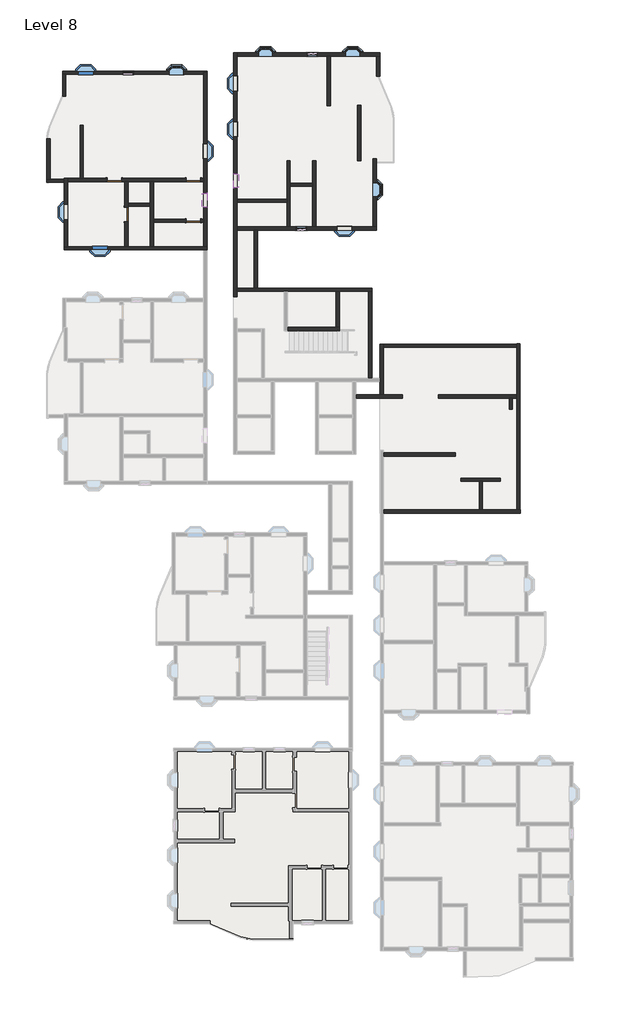
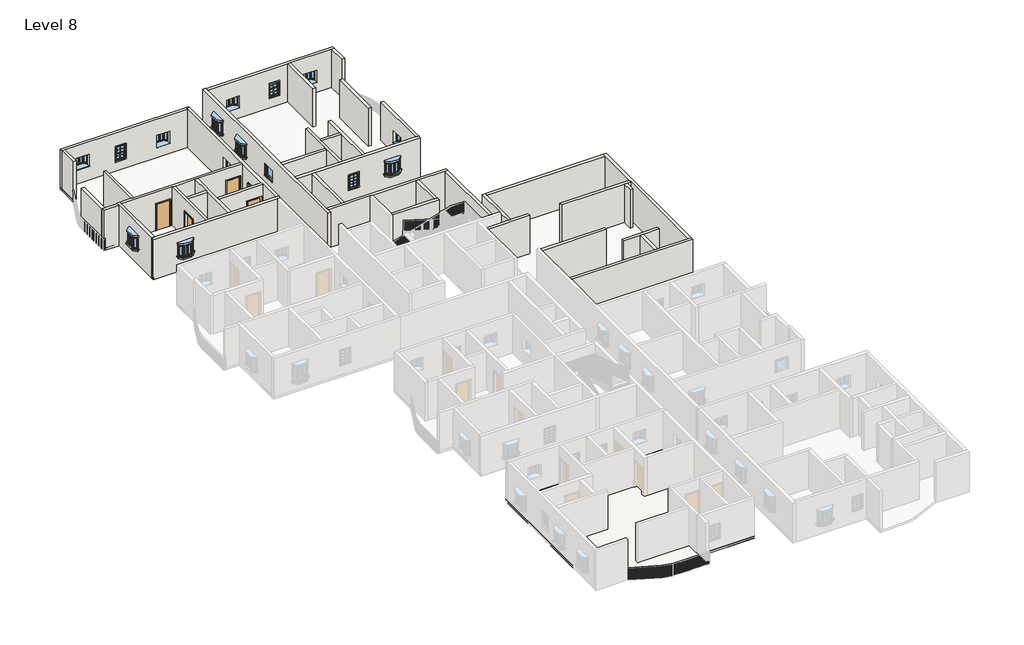
# One storey, part 4 of 14: 39 walls, 16 windows, 4 doors, 2 roofs.
# Revit data of these elements (continued)
# Element 32 (IfcWall, "9\" w") (continued)
#   Top Offset = 0' - 0"
#   Base Offset = 0' - 0"
#   wall height = 10' - 0"
#   Phase Created = New Construction
#   Base Constraint = Level 8
#   Top Constraint = Level 9
#   Materials on its faces: "Default Wall", "Grass"
# Element 33 (IfcWall, "9\" w")
#   Top Offset = 0' - 0"
#   Base Offset = 0' - 0"
#   wall height = 10' - 0"
#   Phase Created = New Construction
#   Base Constraint = Level 8
#   Top Constraint = Level 9
#   Materials on its faces: "Default Wall", "Brick, Soldier Course", "Earth"
# Element 34 (IfcWall, "9\" w")
#   Top Offset = 0' - 0"
#   Base Offset = 0' - 0"
#   wall height = 10' - 0"
#   Phase Created = New Construction
#   Base Constraint = Level 8
#   Top Constraint = Level 9
#   Materials on its faces: "Default Wall", "Earth"
# Element 35 (IfcWall, "9\" w")
#   Top Offset = 0' - 0"
#   Base Offset = 0' - 0"
#   wall height = 10' - 0"
#   Phase Created = New Construction
#   Base Constraint = Level 8
#   Top Constraint = Level 9
#   Materials on its faces: "Default Wall", "Parking Stripe"
# Elements 36, 37, 38 (IfcWall, "9\" w")
#   Top Offset = 0' - 0"
#   Base Offset = 0' - 0"
#   wall height = 10' - 0"
#   Phase Created = New Construction
#   Base Constraint = Level 8
#   Top Constraint = Level 9
#   Materials on its faces: "Default Wall", "Window Frame"
# Element 43 (IfcWall, "9\" w")
#   Top Offset = 0' - 0"
#   Base Offset = 0' - 0"
#   wall height = 10' - 0"
#   Phase Created = New Construction
#   Base Constraint = Level 8
#   Top Constraint = Level 9
#   Materials on its faces: "Default Wall", "Parking Stripe", "Default Mass Interior Wall"
# Element 44 (IfcWall, "9\" w")
#   Top Offset = 0' - 0"
#   Base Offset = 0' - 0"
#   wall height = 10' - 0"
#   Phase Created = New Construction
#   Base Constraint = Level 8
#   Top Constraint = Level 9
#   Materials on its faces: "Default Wall", "Parking Stripe", "Brick, Soldier Course"
# Element 46 (IfcWindow, "910x910mm")
#   Mark = "417"
#   Phase Created = New Construction
#   Materials on its faces: "Window Frame", "Glass"
# Element 47 (IfcWindow, "910x910mm")
#   Mark = "418"
#   Phase Created = New Construction
#   Materials on its faces: "Window Frame", "Glass"
# Element 48 (IfcWindow, "910x910mm")
#   Mark = "419"
#   Phase Created = New Construction
#   Materials on its faces: "Window Frame", "Glass"
# Element 49 (IfcWindow, "910x910mm")
#   Mark = "449"
#   Phase Created = New Construction
#   Materials on its faces: "Window Frame", "Glass"
# Element 50 (IfcWindow, "910x910mm")
#   Mark = "450"
#   Phase Created = New Construction
#   Materials on its faces: "Window Frame", "Glass"
# Element 51 (IfcWindow, "910x910mm")
#   Mark = "478"
#   Phase Created = New Construction
#   Materials on its faces: "Window Frame", "Glass"
# Element 52 (IfcWindow, "910x910mm")
#   Mark = "479"
#   Phase Created = New Construction
#   Materials on its faces: "Window Frame", "Glass"
# Element 53 (IfcWindow, "910x910mm")
#   Mark = "487"
#   Phase Created = New Construction
#   Materials on its faces: "Window Frame", "Glass"
# Element 54 (IfcWindow, "910x910mm")
#   Mark = "488"
#   Phase Created = New Construction
#   Materials on its faces: "Window Frame", "Glass"
# Element 55 (IfcWindow, "910x910mm")
#   Mark = "451"
#   Phase Created = New Construction
#   Materials on its faces: "Window Frame", "Glass"
# Element 56 (IfcWindow, "910x910mm")
#   Mark = "452"
#   Phase Created = New Construction
#   Materials on its faces: "Window Frame", "Glass"
# Element 57 (IfcWindow, "Window-Double-Hung : 26\" x 42\"")
#   Mark = "480"
#   Window Inset = 0' - 0"
#   Interior Wall Closure = 0' - 1 1/2"
#   Frame Extension = 0' - 1 1/4"
#   Exterior Wall Closure = 0' - 0 1/2"
#   Interior Trim Visibility = yes
#   Indicator Visibility = yes
#   Exterior Trim Visibility = yes
#   Phase Created = New Construction
#   Materials on its faces: "Wood - Stained", "Glass", "Clad - White"
# Element 58 (IfcWindow, "Window-Double-Hung : 26\" x 42\"")
#   Mark = "489"
#   Window Inset = 0' - 0"
#   Interior Wall Closure = 0' - 1 1/2"
#   Frame Extension = 0' - 1 1/4"
#   Exterior Wall Closure = 0' - 0 1/2"
#   Interior Trim Visibility = yes
#   Indicator Visibility = yes
#   Exterior Trim Visibility = yes
#   Phase Created = New Construction
#   Materials on its faces: "Wood - Stained", "Glass", "Clad - White"
# Element 59 (IfcWindow, "Window-Double-Hung : 26\" x 42\"")
#   Mark = "470"
#   Window Inset = 0' - 0"
#   Interior Wall Closure = 0' - 1 1/2"
#   Frame Extension = 0' - 1 1/4"
#   Exterior Wall Closure = 0' - 0 1/2"
#   Interior Trim Visibility = yes
#   Indicator Visibility = yes
#   Exterior Trim Visibility = yes
#   Phase Created = New Construction
#   Materials on its faces: "Wood - Stained", "Glass", "Clad - White"
# Element 60 (IfcWindow, "Windows_Sgl_w-Glazing_Bars : 910x910mm")
#   Mark = "453"
#   Phase Created = New Construction
#   Materials on its faces: "Window Frame", "Glass"
# Element 61 (IfcWindow, "Windows_Sgl_w-Glazing_Bars : 910x910mm")
#   Mark = "457"
#   Phase Created = New Construction
#   Materials on its faces: "Window Frame", "Glass"
# Materials
#   "Door - Panel": class "Wood", colour RGB 210 159 95, transparency 0, Cost = 0
#   "Door - Frame": colour RGB 118 70 51, transparency 0, Cost = 0
#   "Window Frame": colour RGB 249 249 249, transparency 0
#   "Glass": class "Glass", colour RGB 0 128 192, transparency 0.75, Description = "Soda Lime Glass", Cost = 0
#   "Wood - Stained": class "Wood", colour RGB 224 178 126, transparency 0, Cost = 0
#   "Clad - White": class "Wood", colour RGB 242 242 238, transparency 0, Cost = 0
#   "Default Roof": colour RGB 88 101 114, transparency 0, Cost = 0
#   "Default Wall": colour RGB 128 128 128, transparency 0, Cost = 0
#   "Grass": class "Generic", colour RGB 104 137 66, transparency 0, Description = "Physical material.", Cost = 0
#   "Parking Stripe": class "Paint", colour RGB 250 250 91, transparency 0, Cost = 0
#   "Carpet (1)": class "Carpet", colour RGB 124 80 67, transparency 0, Description = "Interior finish", Cost = 0
#   "Brick, Soldier Course": class "Masonry", colour RGB 170 98 104, transparency 0, Description = "Common brick soldier coursed", Cost = 0
#   "Default Mass Interior Wall": class "Generic", colour RGB 195 229 126, transparency 0, Cost = 0
#   "Earth": class "Generic", colour RGB 97 75 62, transparency 0, Description = "Soil", Cost = 0
